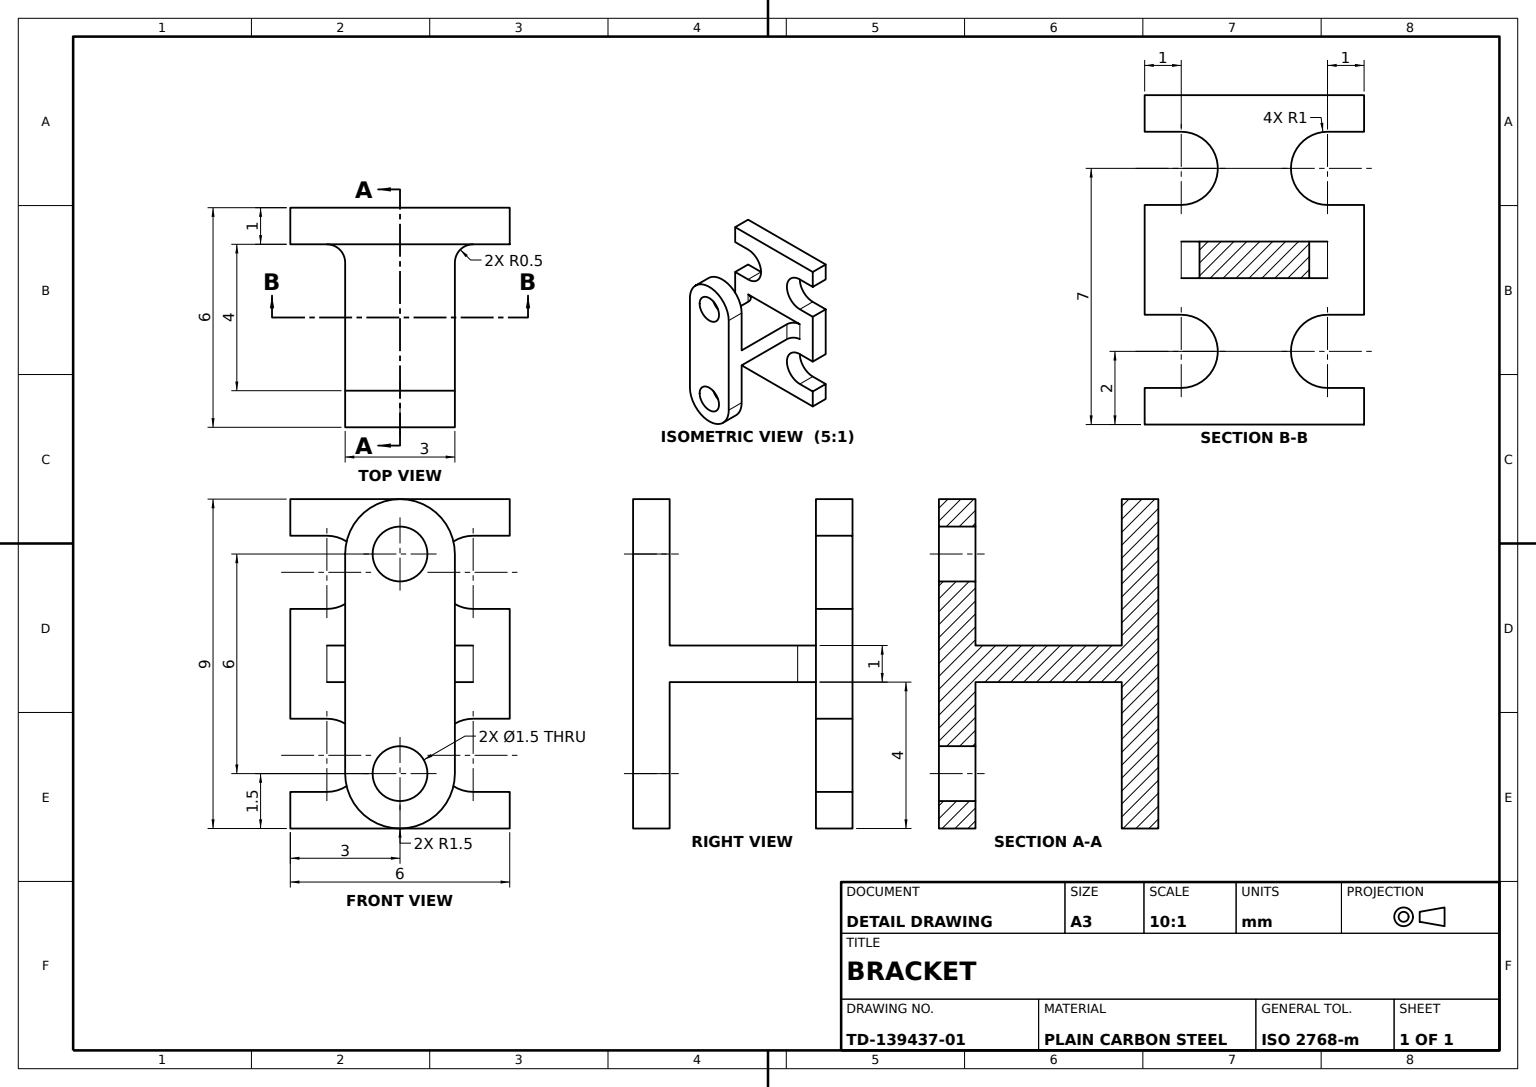
SolidWorks part; units mm, degrees
material "Plain Carbon Steel"
ref_plane "Front Plane" through (0, 0, 0) normal (0, 0, 1) x (1, 0, 0)
ref_plane "Top Plane" through (0, 0, 0) normal (0, 1, 0) x (1, 0, 0)
ref_plane "Right Plane" through (0, 0, 0) normal (1, 0, 0) x (0, 0, -1)
sketch "Base Plate Sketch" plane through (0, 0, 0) normal (0, 0, 1) x (1, 0, 0)
  line L0 (-3, 3.5) -> (-2, 3.5)
  line L1 (-3, 4.5) -> (3, 4.5)
  line L2 (-3, 4.5) -> (-3, 3.5)
  line L3 (-3, -4.5) -> (3, -4.5)
  line L4 (3, 4.5) -> (3, 3.5)
  line L5 (-3, 4.5) -> (3, -4.5) construction
  line L6 (-3, -4.5) -> (3, 4.5) construction
  line L7 (-3, 1.5) -> (-2, 1.5)
  line L8 (-3, -1.5) -> (-2, -1.5)
  line L9 (-3, -3.5) -> (-2, -3.5)
  line L10 (-3, 1.5) -> (-3, -1.5)
  line L11 (3, 1.5) -> (3, -1.5)
  line L12 (3, -3.5) -> (3, -4.5)
  line L13 (-3, -3.5) -> (-3, -4.5)
  line L14 (2, -3.5) -> (3, -3.5)
  line L15 (2, -1.5) -> (3, -1.5)
  line L16 (2, 3.5) -> (3, 3.5)
  line L17 (2, 1.5) -> (3, 1.5)
  arc A0 (-2, 1.5) -> (-2, 3.5) centre (-2, 2.5) ccw
  arc A1 (2, 3.5) -> (2, 1.5) centre (2, 2.5) ccw
  arc A2 (-2, -3.5) -> (-2, -1.5) centre (-2, -2.5) ccw
  arc A3 (2, -1.5) -> (2, -3.5) centre (2, -2.5) ccw
  point P0 (0, 0)
  dimension "D7" = 2
  dimension "D8" = 2
  dimension "D9" = 2
  dimension "D10" = 2
  dimension "D1" = 6
  dimension "D2" = 9
  dimension "D3" = 3
  dimension "D4" = 1.5
  dimension "D5" = 1
  dimension "D6" = 1
  dimension "D11" = 1
  dimension "D12" = 1
  dimension "D13" = 1
  dimension "D14" = 1
extrude "Base Plate" add sketch "Base Plate Sketch" along normal blind 1
sketch "Web Sketch" plane through (0, 0, 1) normal (0, 0, 1) x (1, 0, 0)
  line L1 (1.5, -0.5) -> (-1.5, -0.5)
  line L2 (1.5, -0.5) -> (1.5, 0.5)
  line L3 (1.5, 0.5) -> (-1.5, 0.5)
  line L4 (-1.5, -0.5) -> (-1.5, 0.5)
  line L5 (1.5, -0.5) -> (-1.5, 0.5) construction
  line L6 (1.5, 0.5) -> (-1.5, -0.5) construction
  point P0 (0, 0)
  dimension "D1" = 1
  dimension "D2" = 3
extrude "Web" add sketch "Web Sketch" along normal blind 4
sketch "Link Plate Sketch" plane through (0, 0, 5) normal (0, 0, 1) x (1, 0, 0)
  line L0 (0, 3) -> (0, -3) construction
  line L1 (1.5, 3) -> (1.5, -3)
  line L2 (-1.5, 3) -> (-1.5, -3)
  line L3 (3, 4.5) -> (-3, 4.5) construction
  line L5 (-3, -4.5) -> (3, -4.5) construction
  arc A0 (1.5, 3) -> (-1.5, 3) centre (0, 3) ccw
  arc A1 (-1.5, -3) -> (1.5, -3) centre (0, -3) ccw
  circle A2 centre (0, 3) radius 0.75
  circle A3 centre (0, -3) radius 0.75
  point P3 (0, 0)
  dimension "D1" = 1.5
  dimension "D2" = 1.5
  dimension "D3" = 1.5
extrude "Link Plate" add sketch "Link Plate Sketch" along normal blind 1
fillet "Web Root Fillet R0.5 A" radius 0.5 1 edges at (1.5, 0, 1)
fillet "Web Root Fillet R0.5 B" radius 0.5 1 edges at (-1.5, 0, 1)
